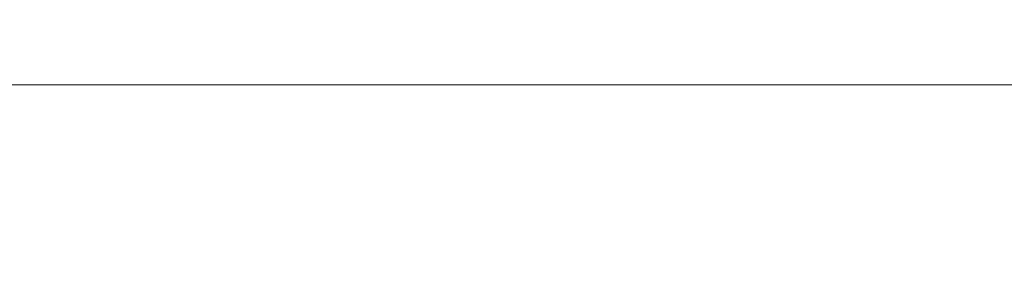
# Model space of a CAD drawing. Units: inches. Extents: x 459864 to 460310, y 324185 to 324787.
# Tile 11 of 112: x 460069.719 to 460071.217, y 324240.835 to 324241.221. Entities that reach past the tile are written whole.
import ezdxf

# ---------------------------------------------------------------- set-up
doc = ezdxf.new("R2010")
doc.units = ezdxf.units.IN
for name, color, linetype, lineweight in [('A-ANNO-DIMS', 2, 'Continuous', 18), ('L-HRDS', 9, 'Continuous', 18), ('L-SITE-PATT', 252, 'Continuous', 13)]:
    doc.layers.add(name, color=color, linetype=linetype, lineweight=lineweight)
doc.styles.get("Standard").update_dxf_attribs({"font": 'arial.ttf'})
doc.dimstyles.new('ISO-25', dxfattribs={"dimtxt": 6, "dimasz": 2.5, "dimexe": 1.25, "dimexo": 0.625, "dimtad": 1, "dimdec": 1, "dimlunit": 3, "dimtxsty": 'Standard', "dimcen": 2.5, "dimadec": 0, "dimazin": 0, "dimtfac": 1, "dimtdec": 1, "dimtmove": 0, "dimatfit": 3, "dimfxl": 1, "dimarcsym": 0})

# ---------------------------------------------------------------- blocks, each defined once
blk = doc.blocks.new('Stepping Stone - hexagonal')
blk.add_line((3.1951, 10.0666), (-5.0989, 10.0666))
blk = doc.blocks.new('*D37')
at = {"layer": 'A-ANNO-DIMS', "color": 0, "lineweight": -2, "transparency": 16777216}
for p, q in [((460077.6779, 324241.1222), (460077.6779, 324260.257)), ((460076.5007, 324241.1222), (460078.9279, 324241.1222)), ((460077.6779, 324231.6078), (460077.6779, 324238.6222)), ((460076.5007, 324229.1078), (460078.9279, 324229.1078))]:
    blk.add_line(p, q, dxfattribs=at)
at = {"layer": 'A-ANNO-DIMS', "color": 0, "transparency": 16777216}
for points in [[(460077.2612, 324238.6222), (460078.0946, 324238.6222), (460077.6779, 324241.1222)], [(460077.2612, 324231.6078), (460078.0946, 324231.6078), (460077.6779, 324229.1078)]]:
    blk.add_solid(points, dxfattribs=at)
at = {"layer": 'Defpoints', "color": 0, "transparency": 16777216}
for p in [(460075.8757, 324241.1222), (460077.6779, 324241.1222), (460075.8757, 324229.1078)]:
    blk.add_point(p, dxfattribs=at)
at = {"layer": 'A-ANNO-DIMS', "color": 0, "transparency": 16777216, "insert": (460073.9895, 324251.9396), "char_height": 6, "attachment_point": 5, "rotation": 90}
blk.add_mtext('1\'-0"', dxfattribs=at)

msp = doc.modelspace()

# ---------------------------------------------------------------- hatches: boundary and pattern name
at = {"layer": 'L-SITE-PATT'}
h = msp.add_hatch(dxfattribs=at)
h.set_pattern_fill('DOTS', color=256)
h.paths.add_polyline_path([(460269.8036, 324283.4832), (460247.1149, 324283.4832), (460121.9293, 324283.4832), (460121.9293, 324252.473), (460117.4293, 324252.473), (460110.1236, 324252.473), (460110.1236, 324243.2865), (460080.8295, 324243.2865), (460080.8295, 324252.473), (460061.1149, 324252.473), (460061.1149, 324251.8824), (460077.9089, 324251.8824), (460077.9089, 324199.4832), (460080.8295, 324199.4832), (460080.8295, 324207.5532), (460110.1236, 324207.5532), (460110.1236, 324199.4832), (460110.8133, 324199.4832), (460262.1149, 324199.4832), (460269.8036, 324199.4832)], flags=17)
edge = h.paths.add_edge_path(flags=0)
edge.add_ellipse((460222.5903, 324263.8132), major_axis=(-8.4853, 8.4853), ratio=1, start_angle=405, end_angle=495, ccw=False)
edge.add_line((460214.8209, 324254.6599), (460214.8316, 324254.6659))
edge.add_ellipse((460222.5903, 324263.8132), major_axis=(-8.4853, 8.4853), ratio=1, start_angle=405, end_angle=495, ccw=False)
edge.add_line((460210.7589, 324261.7806), (460210.7676, 324261.7868))
edge.add_ellipse((460222.5903, 324263.8132), major_axis=(-8.4853, 8.4853), ratio=1, start_angle=405, end_angle=495, ccw=False)
edge.add_ellipse((460222.5903, 324263.8132), major_axis=(-8.4853, 8.4853), ratio=1, start_angle=392.75402, end_angle=405, ccw=False)
edge.add_ellipse((460222.5903, 324263.8132), major_axis=(-8.4853, 8.4853), ratio=1, start_angle=380.93472, end_angle=392.75402, ccw=False)
edge.add_line((460211.3371, 324267.985), (460211.3404, 324267.985))
edge.add_ellipse((460222.5903, 324263.8132), major_axis=(-8.4853, 8.4853), ratio=1, start_angle=380.93472, end_angle=392.75402, ccw=False)
edge.add_ellipse((460222.5903, 324263.8132), major_axis=(-8.4853, 8.4853), ratio=1, start_angle=347.90152, end_angle=380.93472, ccw=False)
edge.add_ellipse((460222.5903, 324263.8132), major_axis=(-8.4853, 8.4853), ratio=1, start_angle=327.06192, end_angle=347.90152, ccw=False)
edge.add_ellipse((460222.5903, 324263.8132), major_axis=(-8.4853, 8.4853), ratio=1, start_angle=278.32464, end_angle=327.06192, ccw=False)
edge.add_line((460225.1583, 324275.536), (460225.1577, 324275.5346))
edge.add_ellipse((460222.5903, 324263.8132), major_axis=(-8.4853, 8.4853), ratio=1, start_angle=278.32464, end_angle=327.06192, ccw=False)
edge.add_ellipse((460222.5903, 324263.8132), major_axis=(-8.4853, 8.4853), ratio=1, start_angle=260.64357, end_angle=278.32464, ccw=False)
edge.add_ellipse((460222.5903, 324263.8132), major_axis=(-8.4853, 8.4853), ratio=1, start_angle=225, end_angle=260.64357, ccw=False)
edge.add_line((460234.5088, 324265.2428), (460234.5015, 324265.2394))
edge.add_ellipse((460222.5903, 324263.8132), major_axis=(-8.4853, 8.4853), ratio=1, start_angle=225, end_angle=260.64357, ccw=False)
edge.add_ellipse((460222.5903, 324263.8132), major_axis=(-8.4853, 8.4853), ratio=1, start_angle=495, end_angle=585, ccw=False)
edge.add_line((460234.4367, 324261.8612), (460234.4238, 324261.8578))
edge.add_ellipse((460222.5903, 324263.8132), major_axis=(-8.4853, 8.4853), ratio=1, start_angle=495, end_angle=585, ccw=False)
edge.add_line((460227.9501, 324253.0672), (460227.9464, 324253.0831))
edge.add_ellipse((460222.5903, 324263.8132), major_axis=(-8.4853, 8.4853), ratio=1, start_angle=495, end_angle=585, ccw=False)
edge.add_line((460226.223, 324252.3693), (460226.211, 324252.3796))
edge.add_ellipse((460222.5903, 324263.8132), major_axis=(-8.4853, 8.4853), ratio=1, start_angle=495, end_angle=585, ccw=False)
h.paths.add_polyline_path([(460219.6515, 324254.3467), (460218.4613, 324253.545), (460218.2754, 324254.7893), (460219.6424, 324256.5418), (460219.6246, 324260.8476), (460216.1101, 324257.333), (460214.35, 324256.9781), (460215.4164, 324259.3557), (460212.5239, 324258.4958), (460213.1373, 324259.9298), (460218.5072, 324263.8132), (460222.5903, 324263.8132), (460222.5903, 324267.8067), (460218.1755, 324272.2123), (460219.026, 324274.639), (460222.5903, 324272.8111), (460222.5903, 324275.4233), (460223.0571, 324274.8249), (460222.6752, 324273.4922), (460225.9117, 324267.1346), (460219.6246, 324260.8476)], flags=0)
edge = h.paths.add_edge_path(flags=0)
edge.add_ellipse((460194.5758, 324264.0465), major_axis=(-8.4853, 8.4853), ratio=1, start_angle=495, end_angle=585, ccw=False)
edge.add_line((460199.9356, 324253.3005), (460199.9319, 324253.3164))
edge.add_ellipse((460194.5758, 324264.0465), major_axis=(-8.4853, 8.4853), ratio=1, start_angle=495, end_angle=585, ccw=False)
edge.add_line((460198.2084, 324252.6025), (460198.1965, 324252.6128))
edge.add_ellipse((460194.5758, 324264.0465), major_axis=(-8.4853, 8.4853), ratio=1, start_angle=495, end_angle=585, ccw=False)
edge.add_ellipse((460194.5758, 324264.0465), major_axis=(-8.4853, 8.4853), ratio=1, start_angle=405, end_angle=495, ccw=False)
edge.add_line((460186.8063, 324254.8932), (460186.8171, 324254.8992))
edge.add_ellipse((460194.5758, 324264.0465), major_axis=(-8.4853, 8.4853), ratio=1, start_angle=405, end_angle=495, ccw=False)
edge.add_line((460182.7444, 324262.0138), (460182.753, 324262.0201))
edge.add_ellipse((460194.5758, 324264.0465), major_axis=(-8.4853, 8.4853), ratio=1, start_angle=405, end_angle=495, ccw=False)
edge.add_ellipse((460194.5758, 324264.0465), major_axis=(-8.4853, 8.4853), ratio=1, start_angle=392.75402, end_angle=405, ccw=False)
edge.add_ellipse((460194.5758, 324264.0465), major_axis=(-8.4853, 8.4853), ratio=1, start_angle=380.93472, end_angle=392.75402, ccw=False)
edge.add_line((460183.3225, 324268.2183), (460183.3259, 324268.2183))
edge.add_ellipse((460194.5758, 324264.0465), major_axis=(-8.4853, 8.4853), ratio=1, start_angle=380.93472, end_angle=392.75402, ccw=False)
edge.add_ellipse((460194.5758, 324264.0465), major_axis=(-8.4853, 8.4853), ratio=1, start_angle=347.90152, end_angle=380.93472, ccw=False)
edge.add_ellipse((460194.5758, 324264.0465), major_axis=(-8.4853, 8.4853), ratio=1, start_angle=327.06192, end_angle=347.90152, ccw=False)
edge.add_ellipse((460194.5758, 324264.0465), major_axis=(-8.4853, 8.4853), ratio=1, start_angle=278.32464, end_angle=327.06192, ccw=False)
edge.add_line((460197.1437, 324275.7693), (460197.1432, 324275.7679))
edge.add_ellipse((460194.5758, 324264.0465), major_axis=(-8.4853, 8.4853), ratio=1, start_angle=278.32464, end_angle=327.06192, ccw=False)
edge.add_ellipse((460194.5758, 324264.0465), major_axis=(-8.4853, 8.4853), ratio=1, start_angle=260.64357, end_angle=278.32464, ccw=False)
edge.add_ellipse((460194.5758, 324264.0465), major_axis=(-8.4853, 8.4853), ratio=1, start_angle=225, end_angle=260.64357, ccw=False)
edge.add_line((460206.4943, 324265.4761), (460206.4869, 324265.4727))
edge.add_ellipse((460194.5758, 324264.0465), major_axis=(-8.4853, 8.4853), ratio=1, start_angle=225, end_angle=260.64357, ccw=False)
edge.add_ellipse((460194.5758, 324264.0465), major_axis=(-8.4853, 8.4853), ratio=1, start_angle=495, end_angle=585, ccw=False)
edge.add_line((460206.4221, 324262.0945), (460206.4092, 324262.0911))
h.paths.add_polyline_path([(460191.6101, 324261.0808), (460191.6369, 324254.5799), (460190.4468, 324253.7783), (460190.2609, 324255.0226), (460191.6279, 324256.775), (460191.6101, 324261.0808), (460188.0956, 324257.5663), (460186.3354, 324257.2113), (460187.4018, 324259.5889), (460184.5094, 324258.7291), (460185.1228, 324260.1631), (460190.4927, 324264.0465), (460194.5758, 324264.0465), (460194.5758, 324268.04), (460190.161, 324272.4456), (460191.0114, 324274.8722), (460194.5758, 324273.0444), (460194.5758, 324275.6566), (460195.0426, 324275.0582), (460194.6607, 324273.7255), (460197.8971, 324267.3679)], flags=0)
edge = h.paths.add_edge_path(flags=0)
edge.add_ellipse((460252.912, 324263.5776), major_axis=(-8.4853, 8.4853), ratio=1, start_angle=405, end_angle=495, ccw=False)
edge.add_line((460241.0806, 324261.5449), (460241.0892, 324261.5512))
edge.add_ellipse((460252.912, 324263.5776), major_axis=(-8.4853, 8.4853), ratio=1, start_angle=405, end_angle=495, ccw=False)
edge.add_ellipse((460252.912, 324263.5776), major_axis=(-8.4853, 8.4853), ratio=1, start_angle=392.75402, end_angle=405, ccw=False)
edge.add_ellipse((460252.912, 324263.5776), major_axis=(-8.4853, 8.4853), ratio=1, start_angle=380.93472, end_angle=392.75402, ccw=False)
edge.add_line((460241.6587, 324267.7494), (460241.6621, 324267.7494))
edge.add_ellipse((460252.912, 324263.5776), major_axis=(-8.4853, 8.4853), ratio=1, start_angle=380.93472, end_angle=392.75402, ccw=False)
edge.add_ellipse((460252.912, 324263.5776), major_axis=(-8.4853, 8.4853), ratio=1, start_angle=347.90152, end_angle=380.93472, ccw=False)
edge.add_ellipse((460252.912, 324263.5776), major_axis=(-8.4853, 8.4853), ratio=1, start_angle=327.06192, end_angle=347.90152, ccw=False)
edge.add_ellipse((460252.912, 324263.5776), major_axis=(-8.4853, 8.4853), ratio=1, start_angle=278.32464, end_angle=327.06192, ccw=False)
edge.add_line((460255.4799, 324275.3004), (460255.4794, 324275.299))
edge.add_ellipse((460252.912, 324263.5776), major_axis=(-8.4853, 8.4853), ratio=1, start_angle=278.32464, end_angle=327.06192, ccw=False)
edge.add_ellipse((460252.912, 324263.5776), major_axis=(-8.4853, 8.4853), ratio=1, start_angle=260.64357, end_angle=278.32464, ccw=False)
edge.add_ellipse((460252.912, 324263.5776), major_axis=(-8.4853, 8.4853), ratio=1, start_angle=225, end_angle=260.64357, ccw=False)
edge.add_line((460264.8305, 324265.0072), (460264.8231, 324265.0038))
edge.add_ellipse((460252.912, 324263.5776), major_axis=(-8.4853, 8.4853), ratio=1, start_angle=225, end_angle=260.64357, ccw=False)
edge.add_ellipse((460252.912, 324263.5776), major_axis=(-8.4853, 8.4853), ratio=1, start_angle=495, end_angle=585, ccw=False)
edge.add_line((460264.7583, 324261.6256), (460264.7454, 324261.6222))
edge.add_ellipse((460252.912, 324263.5776), major_axis=(-8.4853, 8.4853), ratio=1, start_angle=495, end_angle=585, ccw=False)
edge.add_line((460258.2718, 324252.8316), (460258.2681, 324252.8475))
edge.add_ellipse((460252.912, 324263.5776), major_axis=(-8.4853, 8.4853), ratio=1, start_angle=495, end_angle=585, ccw=False)
edge.add_line((460256.5446, 324252.1337), (460256.5327, 324252.1439))
edge.add_ellipse((460252.912, 324263.5776), major_axis=(-8.4853, 8.4853), ratio=1, start_angle=495, end_angle=585, ccw=False)
edge.add_ellipse((460252.912, 324263.5776), major_axis=(-8.4853, 8.4853), ratio=1, start_angle=405, end_angle=495, ccw=False)
edge.add_line((460245.1425, 324254.4243), (460245.1533, 324254.4303))
h.paths.add_polyline_path([(460244.6716, 324256.7425), (460245.738, 324259.1201), (460242.8456, 324258.2602), (460243.459, 324259.6942), (460248.8289, 324263.5776), (460252.912, 324263.5776), (460252.912, 324267.5711), (460248.4972, 324271.9767), (460249.3476, 324274.4034), (460252.912, 324272.5755), (460252.912, 324275.1877), (460253.3788, 324274.5893), (460252.9969, 324273.2566), (460256.2333, 324266.899), (460249.9463, 324260.612), (460249.9731, 324254.111), (460248.783, 324253.3094), (460248.5971, 324254.5537), (460249.9641, 324256.3062), (460249.9463, 324260.612), (460246.4318, 324257.0974)], flags=0)
edge = h.paths.add_edge_path(flags=0)
edge.add_ellipse((460167.4387, 324262.8328), major_axis=(-8.4853, 8.4853), ratio=1, start_angle=495, end_angle=585, ccw=False)
edge.add_line((460172.7985, 324252.0868), (460172.7948, 324252.1027))
edge.add_ellipse((460167.4387, 324262.8328), major_axis=(-8.4853, 8.4853), ratio=1, start_angle=495, end_angle=585, ccw=False)
edge.add_line((460171.0714, 324251.3888), (460171.0594, 324251.3991))
edge.add_ellipse((460167.4387, 324262.8328), major_axis=(-8.4853, 8.4853), ratio=1, start_angle=495, end_angle=585, ccw=False)
edge.add_ellipse((460167.4387, 324262.8328), major_axis=(-8.4853, 8.4853), ratio=1, start_angle=405, end_angle=495, ccw=False)
edge.add_line((460159.6693, 324253.6795), (460159.68, 324253.6855))
edge.add_ellipse((460167.4387, 324262.8328), major_axis=(-8.4853, 8.4853), ratio=1, start_angle=405, end_angle=495, ccw=False)
edge.add_line((460155.6073, 324260.8001), (460155.616, 324260.8064))
edge.add_ellipse((460167.4387, 324262.8328), major_axis=(-8.4853, 8.4853), ratio=1, start_angle=405, end_angle=495, ccw=False)
edge.add_ellipse((460167.4387, 324262.8328), major_axis=(-8.4853, 8.4853), ratio=1, start_angle=392.75402, end_angle=405, ccw=False)
edge.add_ellipse((460167.4387, 324262.8328), major_axis=(-8.4853, 8.4853), ratio=1, start_angle=380.93472, end_angle=392.75402, ccw=False)
edge.add_line((460156.1855, 324267.0046), (460156.1888, 324267.0046))
edge.add_ellipse((460167.4387, 324262.8328), major_axis=(-8.4853, 8.4853), ratio=1, start_angle=380.93472, end_angle=392.75402, ccw=False)
edge.add_ellipse((460167.4387, 324262.8328), major_axis=(-8.4853, 8.4853), ratio=1, start_angle=347.90152, end_angle=380.93472, ccw=False)
edge.add_ellipse((460167.4387, 324262.8328), major_axis=(-8.4853, 8.4853), ratio=1, start_angle=327.06192, end_angle=347.90152, ccw=False)
edge.add_ellipse((460167.4387, 324262.8328), major_axis=(-8.4853, 8.4853), ratio=1, start_angle=278.32464, end_angle=327.06192, ccw=False)
edge.add_line((460170.0067, 324274.5556), (460170.0061, 324274.5542))
edge.add_ellipse((460167.4387, 324262.8328), major_axis=(-8.4853, 8.4853), ratio=1, start_angle=278.32464, end_angle=327.06192, ccw=False)
edge.add_ellipse((460167.4387, 324262.8328), major_axis=(-8.4853, 8.4853), ratio=1, start_angle=260.64357, end_angle=278.32464, ccw=False)
edge.add_ellipse((460167.4387, 324262.8328), major_axis=(-8.4853, 8.4853), ratio=1, start_angle=225, end_angle=260.64357, ccw=False)
edge.add_line((460179.3572, 324264.2624), (460179.3499, 324264.259))
edge.add_ellipse((460167.4387, 324262.8328), major_axis=(-8.4853, 8.4853), ratio=1, start_angle=225, end_angle=260.64357, ccw=False)
edge.add_ellipse((460167.4387, 324262.8328), major_axis=(-8.4853, 8.4853), ratio=1, start_angle=495, end_angle=585, ccw=False)
edge.add_line((460179.2851, 324260.8808), (460179.2722, 324260.8774))
h.paths.add_polyline_path([(460164.473, 324259.8671), (460164.4998, 324253.3662), (460163.3097, 324252.5645), (460163.1238, 324253.8089), (460164.4908, 324255.5613), (460164.473, 324259.8671), (460160.9585, 324256.3526), (460159.1984, 324255.9976), (460160.2648, 324258.3752), (460157.3723, 324257.5154), (460157.9857, 324258.9494), (460163.3556, 324262.8328), (460167.4387, 324262.8328), (460167.4387, 324266.8263), (460163.0239, 324271.2319), (460163.8744, 324273.6585), (460167.4387, 324271.8307), (460167.4387, 324274.4429), (460167.9055, 324273.8445), (460167.5236, 324272.5118), (460170.7601, 324266.1542)], flags=0)
edge = h.paths.add_edge_path(flags=0)
edge.add_ellipse((460140.7581, 324262.3696), major_axis=(-8.4853, 8.4853), ratio=1, start_angle=495, end_angle=585, ccw=False)
edge.add_line((460146.1179, 324251.6235), (460146.1142, 324251.6395))
edge.add_ellipse((460140.7581, 324262.3696), major_axis=(-8.4853, 8.4853), ratio=1, start_angle=495, end_angle=585, ccw=False)
edge.add_line((460144.3908, 324250.9256), (460144.3788, 324250.9359))
edge.add_ellipse((460140.7581, 324262.3696), major_axis=(-8.4853, 8.4853), ratio=1, start_angle=495, end_angle=585, ccw=False)
edge.add_ellipse((460140.7581, 324262.3696), major_axis=(-8.4853, 8.4853), ratio=1, start_angle=405, end_angle=495, ccw=False)
edge.add_line((460132.9887, 324253.2162), (460132.9994, 324253.2223))
edge.add_ellipse((460140.7581, 324262.3696), major_axis=(-8.4853, 8.4853), ratio=1, start_angle=405, end_angle=495, ccw=False)
edge.add_line((460128.9267, 324260.3369), (460128.9354, 324260.3432))
edge.add_ellipse((460140.7581, 324262.3696), major_axis=(-8.4853, 8.4853), ratio=1, start_angle=405, end_angle=495, ccw=False)
edge.add_ellipse((460140.7581, 324262.3696), major_axis=(-8.4853, 8.4853), ratio=1, start_angle=392.75402, end_angle=405, ccw=False)
edge.add_ellipse((460140.7581, 324262.3696), major_axis=(-8.4853, 8.4853), ratio=1, start_angle=380.93472, end_angle=392.75402, ccw=False)
edge.add_line((460129.5049, 324266.5414), (460129.5082, 324266.5414))
edge.add_ellipse((460140.7581, 324262.3696), major_axis=(-8.4853, 8.4853), ratio=1, start_angle=380.93472, end_angle=392.75402, ccw=False)
edge.add_ellipse((460140.7581, 324262.3696), major_axis=(-8.4853, 8.4853), ratio=1, start_angle=347.90152, end_angle=380.93472, ccw=False)
edge.add_ellipse((460140.7581, 324262.3696), major_axis=(-8.4853, 8.4853), ratio=1, start_angle=327.06192, end_angle=347.90152, ccw=False)
edge.add_ellipse((460140.7581, 324262.3696), major_axis=(-8.4853, 8.4853), ratio=1, start_angle=278.32464, end_angle=327.06192, ccw=False)
edge.add_line((460143.3261, 324274.0923), (460143.3255, 324274.091))
edge.add_ellipse((460140.7581, 324262.3696), major_axis=(-8.4853, 8.4853), ratio=1, start_angle=278.32464, end_angle=327.06192, ccw=False)
edge.add_ellipse((460140.7581, 324262.3696), major_axis=(-8.4853, 8.4853), ratio=1, start_angle=260.64357, end_angle=278.32464, ccw=False)
edge.add_ellipse((460140.7581, 324262.3696), major_axis=(-8.4853, 8.4853), ratio=1, start_angle=225, end_angle=260.64357, ccw=False)
edge.add_line((460152.6766, 324263.7992), (460152.6692, 324263.7958))
edge.add_ellipse((460140.7581, 324262.3696), major_axis=(-8.4853, 8.4853), ratio=1, start_angle=225, end_angle=260.64357, ccw=False)
edge.add_ellipse((460140.7581, 324262.3696), major_axis=(-8.4853, 8.4853), ratio=1, start_angle=495, end_angle=585, ccw=False)
edge.add_line((460152.6045, 324260.4176), (460152.5916, 324260.4142))
h.paths.add_polyline_path([(460137.7924, 324259.4039), (460137.8192, 324252.903), (460136.6291, 324252.1013), (460136.4432, 324253.3457), (460137.8102, 324255.0981), (460137.7924, 324259.4039), (460134.2779, 324255.8894), (460132.5178, 324255.5344), (460133.5842, 324257.912), (460130.6917, 324257.0522), (460131.3051, 324258.4862), (460136.675, 324262.3696), (460140.7581, 324262.3696), (460140.7581, 324266.3631), (460136.3433, 324270.7687), (460137.1938, 324273.1953), (460140.7581, 324271.3675), (460140.7581, 324273.9797), (460141.2249, 324273.3813), (460140.843, 324272.0486), (460144.0795, 324265.691)], flags=0)
h.paths.add_polyline_path([(460110.1236, 324227.4139), (460080.8295, 324227.4139), (460080.8295, 324235.4839), (460110.1236, 324235.4839)], flags=16)
h.paths.add_polyline_path([(460110.1236, 324220.7966), (460110.1236, 324212.7267), (460080.8295, 324212.7267), (460080.8295, 324220.7966)], flags=16)
h.paths.add_polyline_path([(460269.8036, 324283.4832), (460247.1149, 324283.4832), (460121.9293, 324283.4832), (460121.9293, 324252.473), (460117.4293, 324252.473), (460110.1236, 324252.473), (460110.1236, 324243.2865), (460080.8295, 324243.2865), (460080.8295, 324252.473), (460061.1149, 324252.473), (460061.1149, 324251.8824), (460077.9089, 324251.8824), (460077.9089, 324199.4832), (460080.8295, 324199.4832), (460080.8295, 324207.5532), (460110.1236, 324207.5532), (460110.1236, 324199.4832), (460262.1149, 324199.4832), (460269.8036, 324199.4832)], flags=17)
h.paths.add_polyline_path([(460219.6515, 324254.3467), (460218.4613, 324253.545), (460218.2754, 324254.7893), (460219.6424, 324256.5418), (460219.6246, 324260.8476), (460216.1101, 324257.333), (460214.35, 324256.9781), (460215.4164, 324259.3557), (460212.5239, 324258.4958), (460213.1373, 324259.9298), (460218.5072, 324263.8132), (460222.5903, 324263.8132), (460220.1805, 324266.223), (460215.461, 324265.3076), (460211.8345, 324266.1366), (460216.2466, 324267.985), (460218.4185, 324267.985), (460222.5903, 324263.8132), (460222.5903, 324267.8067), (460218.1755, 324272.2123), (460219.026, 324274.639), (460222.5903, 324272.8111), (460222.5903, 324275.4233), (460223.0571, 324274.8249), (460222.6752, 324273.4922), (460225.9117, 324267.1346), (460222.5903, 324263.8132), (460231.3829, 324263.8132), (460228.4847, 324262.4878), (460224.4252, 324261.9783), (460228.6799, 324257.7236), (460228.9658, 324254.791), (460227.1418, 324256.5366), (460227.5421, 324254.8186), (460227.3333, 324253.6145), (460222.5903, 324259.9846), (460222.5903, 324255.4967), (460221.3774, 324256.5408), (460220.5758, 324261.7987), (460219.6246, 324260.8476)], flags=0)
h.paths.add_polyline_path([(460199.1272, 324256.7699), (460199.5275, 324255.0518), (460199.3188, 324253.8477), (460194.5758, 324260.2179), (460194.5758, 324255.7299), (460193.3629, 324256.7741), (460192.5613, 324262.032), (460191.6101, 324261.0808), (460191.6369, 324254.5799), (460190.4468, 324253.7783), (460190.2609, 324255.0226), (460191.6279, 324256.775), (460191.6101, 324261.0808), (460188.0956, 324257.5663), (460186.3354, 324257.2113), (460187.4018, 324259.5889), (460184.5094, 324258.7291), (460185.1228, 324260.1631), (460190.4927, 324264.0465), (460194.5758, 324264.0465), (460192.1659, 324266.4563), (460187.4464, 324265.5409), (460183.82, 324266.3698), (460188.2321, 324268.2183), (460190.404, 324268.2183), (460194.5758, 324264.0465), (460194.5758, 324268.04), (460190.161, 324272.4456), (460191.0114, 324274.8722), (460194.5758, 324273.0444), (460194.5758, 324275.6566), (460195.0426, 324275.0582), (460194.6607, 324273.7255), (460197.8971, 324267.3679), (460194.5758, 324264.0465), (460203.3683, 324264.0465), (460200.4702, 324262.7211), (460196.4107, 324262.2116), (460200.6654, 324257.9569), (460200.9513, 324255.0243)], flags=0)
h.paths.add_polyline_path([(460244.6716, 324256.7425), (460245.738, 324259.1201), (460242.8456, 324258.2602), (460243.459, 324259.6942), (460248.8289, 324263.5776), (460252.912, 324263.5776), (460250.5022, 324265.9874), (460245.7826, 324265.072), (460242.1562, 324265.9009), (460246.5683, 324267.7494), (460248.7402, 324267.7494), (460252.912, 324263.5776), (460252.912, 324267.5711), (460248.4972, 324271.9767), (460249.3476, 324274.4034), (460252.912, 324272.5755), (460252.912, 324275.1877), (460253.3788, 324274.5893), (460252.9969, 324273.2566), (460256.2333, 324266.899), (460252.912, 324263.5776), (460261.7045, 324263.5776), (460258.8064, 324262.2522), (460254.7469, 324261.7427), (460259.0016, 324257.488), (460259.2875, 324254.5554), (460257.4634, 324256.301), (460257.8637, 324254.583), (460257.655, 324253.3789), (460252.912, 324259.749), (460252.912, 324255.2611), (460251.6991, 324256.3052), (460250.8975, 324261.5631), (460249.9463, 324260.612), (460249.9731, 324254.111), (460248.783, 324253.3094), (460248.5971, 324254.5537), (460249.9641, 324256.3062), (460249.9463, 324260.612), (460246.4318, 324257.0974)], flags=0)
h.paths.add_polyline_path([(460173.5283, 324256.7432), (460173.8142, 324253.8106), (460171.9902, 324255.5562), (460172.3905, 324253.8381), (460172.1817, 324252.634), (460167.4387, 324259.0042), (460167.4387, 324254.5162), (460166.2258, 324255.5604), (460165.4242, 324260.8183), (460164.473, 324259.8671), (460164.4998, 324253.3662), (460163.3097, 324252.5645), (460163.1238, 324253.8089), (460164.4908, 324255.5613), (460164.473, 324259.8671), (460160.9585, 324256.3526), (460159.1984, 324255.9976), (460160.2648, 324258.3752), (460157.3723, 324257.5154), (460157.9857, 324258.9494), (460163.3556, 324262.8328), (460167.4387, 324262.8328), (460165.0289, 324265.2426), (460160.3094, 324264.3272), (460156.6829, 324265.1561), (460161.095, 324267.0046), (460163.2669, 324267.0046), (460167.4387, 324262.8328), (460167.4387, 324266.8263), (460163.0239, 324271.2319), (460163.8744, 324273.6585), (460167.4387, 324271.8307), (460167.4387, 324274.4429), (460167.9055, 324273.8445), (460167.5236, 324272.5118), (460170.7601, 324266.1542), (460167.4387, 324262.8328), (460176.2313, 324262.8328), (460173.3331, 324261.5074), (460169.2736, 324260.9979)], flags=0)
h.paths.add_polyline_path([(460146.8477, 324256.28), (460147.1336, 324253.3474), (460145.3096, 324255.093), (460145.7099, 324253.3749), (460145.5011, 324252.1708), (460140.7581, 324258.541), (460140.7581, 324254.053), (460139.5452, 324255.0972), (460138.7436, 324260.3551), (460137.7924, 324259.4039), (460137.8192, 324252.903), (460136.6291, 324252.1013), (460136.4432, 324253.3457), (460137.8102, 324255.0981), (460137.7924, 324259.4039), (460134.2779, 324255.8894), (460132.5178, 324255.5344), (460133.5842, 324257.912), (460130.6917, 324257.0522), (460131.3051, 324258.4862), (460136.675, 324262.3696), (460140.7581, 324262.3696), (460138.3483, 324264.7794), (460133.6288, 324263.864), (460130.0023, 324264.6929), (460134.4144, 324266.5414), (460136.5863, 324266.5414), (460140.7581, 324262.3696), (460140.7581, 324266.3631), (460136.3433, 324270.7687), (460137.1938, 324273.1953), (460140.7581, 324271.3675), (460140.7581, 324273.9797), (460141.2249, 324273.3813), (460140.843, 324272.0486), (460144.0795, 324265.691), (460140.7581, 324262.3696), (460149.5507, 324262.3696), (460146.6525, 324261.0442), (460142.593, 324260.5347)], flags=0)
edge = h.paths.add_edge_path()
edge.add_line((460269.8036, 324272.5491), (460260.8815, 324272.5491))
edge.add_ellipse((460252.912, 324263.5776), major_axis=(-8.4853, 8.4853), ratio=1, start_angle=260.64357, end_angle=273.38462, ccw=False)
edge.add_line((460262.2826, 324271.0921), (460262.2606, 324271.0911))
edge.add_ellipse((460252.912, 324263.5776), major_axis=(-8.4853, 8.4853), ratio=1, start_angle=260.64357, end_angle=273.38462, ccw=False)
edge.add_ellipse((460252.912, 324263.5776), major_axis=(-8.4853, 8.4853), ratio=1, start_angle=225, end_angle=260.64357, ccw=False)
edge.add_line((460263.6086, 324269.0633), (460263.5717, 324269.0583))
edge.add_ellipse((460252.912, 324263.5776), major_axis=(-8.4853, 8.4853), ratio=1, start_angle=225, end_angle=260.64357, ccw=False)
edge.add_line((460264.6155, 324266.3055), (460264.5854, 324266.3052))
edge.add_ellipse((460252.912, 324263.5776), major_axis=(-8.4853, 8.4853), ratio=1, start_angle=225, end_angle=260.64357, ccw=False)
edge.add_line((460264.8305, 324265.0072), (460264.8231, 324265.0038))
edge.add_ellipse((460252.912, 324263.5776), major_axis=(-8.4853, 8.4853), ratio=1, start_angle=225, end_angle=260.64357, ccw=False)
edge.add_ellipse((460252.912, 324263.5776), major_axis=(-8.4853, 8.4853), ratio=1, start_angle=495, end_angle=585, ccw=False)
edge.add_line((460264.7583, 324261.6256), (460264.7454, 324261.6222))
edge.add_ellipse((460252.912, 324263.5776), major_axis=(-8.4853, 8.4853), ratio=1, start_angle=495, end_angle=585, ccw=False)
edge.add_line((460263.4422, 324257.739), (460263.3893, 324257.7792))
edge.add_ellipse((460252.912, 324263.5776), major_axis=(-8.4853, 8.4853), ratio=1, start_angle=495, end_angle=585, ccw=False)
edge.add_line((460258.1281, 324252.7435), (460258.1019, 324252.7787))
edge.add_ellipse((460252.912, 324263.5776), major_axis=(-8.4853, 8.4853), ratio=1, start_angle=495, end_angle=585, ccw=False)
edge.add_line((460256.5446, 324252.1337), (460256.5327, 324252.1439))
edge.add_ellipse((460252.912, 324263.5776), major_axis=(-8.4853, 8.4853), ratio=1, start_angle=495, end_angle=585, ccw=False)
edge.add_ellipse((460252.912, 324263.5776), major_axis=(-8.4853, 8.4853), ratio=1, start_angle=405, end_angle=495, ccw=False)
edge.add_line((460250.594, 324251.7804), (460250.6047, 324251.8198))
edge.add_ellipse((460252.912, 324263.5776), major_axis=(-8.4853, 8.4853), ratio=1, start_angle=405, end_angle=495, ccw=False)
edge.add_line((460245.1425, 324254.4243), (460245.1533, 324254.4303))
edge.add_ellipse((460252.912, 324263.5776), major_axis=(-8.4853, 8.4853), ratio=1, start_angle=405, end_angle=495, ccw=False)
edge.add_line((460243.5246, 324256.059), (460243.5603, 324256.0914))
edge.add_ellipse((460252.912, 324263.5776), major_axis=(-8.4853, 8.4853), ratio=1, start_angle=405, end_angle=495, ccw=False)
edge.add_line((460241.4401, 324259.8927), (460241.5224, 324259.8959))
edge.add_ellipse((460252.912, 324263.5776), major_axis=(-8.4853, 8.4853), ratio=1, start_angle=405, end_angle=495, ccw=False)
edge.add_line((460241.0806, 324261.5449), (460241.0892, 324261.5512))
edge.add_ellipse((460252.912, 324263.5776), major_axis=(-8.4853, 8.4853), ratio=1, start_angle=405, end_angle=495, ccw=False)
edge.add_ellipse((460252.912, 324263.5776), major_axis=(-8.4853, 8.4853), ratio=1, start_angle=392.75402, end_angle=405, ccw=False)
edge.add_line((460241.0503, 324265.4376), (460241.0626, 324265.4428))
edge.add_ellipse((460252.912, 324263.5776), major_axis=(-8.4853, 8.4853), ratio=1, start_angle=392.75402, end_angle=405, ccw=False)
edge.add_ellipse((460252.912, 324263.5776), major_axis=(-8.4853, 8.4853), ratio=1, start_angle=380.93472, end_angle=392.75402, ccw=False)
edge.add_line((460241.4519, 324267.1764), (460241.469, 324267.171))
edge.add_ellipse((460252.912, 324263.5776), major_axis=(-8.4853, 8.4853), ratio=1, start_angle=380.93472, end_angle=392.75402, ccw=False)
edge.add_line((460241.6587, 324267.7494), (460241.6621, 324267.7494))
edge.add_ellipse((460252.912, 324263.5776), major_axis=(-8.4853, 8.4853), ratio=1, start_angle=380.93472, end_angle=392.75402, ccw=False)
edge.add_ellipse((460252.912, 324263.5776), major_axis=(-8.4853, 8.4853), ratio=1, start_angle=356.61538, end_angle=380.93472, ccw=False)
edge.add_line((460244.8803, 324272.4877), (460244.7127, 324272.5491))
edge.add_line((460244.7127, 324272.5491), (460230.8174, 324272.5491))
edge.add_ellipse((460222.5903, 324263.8132), major_axis=(-8.4853, 8.4853), ratio=1, start_angle=260.64357, end_angle=271.71777, ccw=False)
edge.add_ellipse((460222.5903, 324263.8132), major_axis=(-8.4853, 8.4853), ratio=1, start_angle=225, end_angle=260.64357, ccw=False)
edge.add_line((460233.2869, 324269.2989), (460233.25, 324269.2939))
edge.add_ellipse((460222.5903, 324263.8132), major_axis=(-8.4853, 8.4853), ratio=1, start_angle=225, end_angle=260.64357, ccw=False)
edge.add_line((460234.2938, 324266.5412), (460234.2637, 324266.5408))
edge.add_ellipse((460222.5903, 324263.8132), major_axis=(-8.4853, 8.4853), ratio=1, start_angle=225, end_angle=260.64357, ccw=False)
edge.add_line((460234.5088, 324265.2428), (460234.5015, 324265.2394))
edge.add_ellipse((460222.5903, 324263.8132), major_axis=(-8.4853, 8.4853), ratio=1, start_angle=225, end_angle=260.64357, ccw=False)
edge.add_ellipse((460222.5903, 324263.8132), major_axis=(-8.4853, 8.4853), ratio=1, start_angle=495, end_angle=585, ccw=False)
edge.add_line((460234.4367, 324261.8612), (460234.4238, 324261.8578))
edge.add_ellipse((460222.5903, 324263.8132), major_axis=(-8.4853, 8.4853), ratio=1, start_angle=495, end_angle=585, ccw=False)
edge.add_line((460233.1205, 324257.9746), (460233.0676, 324258.0149))
edge.add_ellipse((460222.5903, 324263.8132), major_axis=(-8.4853, 8.4853), ratio=1, start_angle=495, end_angle=585, ccw=False)
edge.add_line((460227.8064, 324252.9791), (460227.7802, 324253.0143))
edge.add_ellipse((460222.5903, 324263.8132), major_axis=(-8.4853, 8.4853), ratio=1, start_angle=495, end_angle=585, ccw=False)
edge.add_line((460226.223, 324252.3693), (460226.211, 324252.3796))
edge.add_ellipse((460222.5903, 324263.8132), major_axis=(-8.4853, 8.4853), ratio=1, start_angle=495, end_angle=585, ccw=False)
edge.add_ellipse((460222.5903, 324263.8132), major_axis=(-8.4853, 8.4853), ratio=1, start_angle=405, end_angle=495, ccw=False)
edge.add_line((460220.2723, 324252.016), (460220.283, 324252.0554))
edge.add_ellipse((460222.5903, 324263.8132), major_axis=(-8.4853, 8.4853), ratio=1, start_angle=405, end_angle=495, ccw=False)
edge.add_line((460214.8209, 324254.6599), (460214.8316, 324254.6659))
edge.add_ellipse((460222.5903, 324263.8132), major_axis=(-8.4853, 8.4853), ratio=1, start_angle=405, end_angle=495, ccw=False)
edge.add_line((460213.2029, 324256.2946), (460213.2387, 324256.327))
edge.add_ellipse((460222.5903, 324263.8132), major_axis=(-8.4853, 8.4853), ratio=1, start_angle=405, end_angle=495, ccw=False)
edge.add_line((460211.1184, 324260.1283), (460211.2008, 324260.1315))
edge.add_ellipse((460222.5903, 324263.8132), major_axis=(-8.4853, 8.4853), ratio=1, start_angle=405, end_angle=495, ccw=False)
edge.add_line((460210.7589, 324261.7806), (460210.7676, 324261.7868))
edge.add_ellipse((460222.5903, 324263.8132), major_axis=(-8.4853, 8.4853), ratio=1, start_angle=405, end_angle=495, ccw=False)
edge.add_ellipse((460222.5903, 324263.8132), major_axis=(-8.4853, 8.4853), ratio=1, start_angle=392.75402, end_angle=405, ccw=False)
edge.add_line((460210.7286, 324265.6732), (460210.7409, 324265.6784))
edge.add_ellipse((460222.5903, 324263.8132), major_axis=(-8.4853, 8.4853), ratio=1, start_angle=392.75402, end_angle=405, ccw=False)
edge.add_ellipse((460222.5903, 324263.8132), major_axis=(-8.4853, 8.4853), ratio=1, start_angle=380.93472, end_angle=392.75402, ccw=False)
edge.add_line((460211.1302, 324267.412), (460211.1474, 324267.4066))
edge.add_ellipse((460222.5903, 324263.8132), major_axis=(-8.4853, 8.4853), ratio=1, start_angle=380.93472, end_angle=392.75402, ccw=False)
edge.add_line((460211.3371, 324267.985), (460211.3404, 324267.985))
edge.add_ellipse((460222.5903, 324263.8132), major_axis=(-8.4853, 8.4853), ratio=1, start_angle=380.93472, end_angle=392.75402, ccw=False)
edge.add_ellipse((460222.5903, 324263.8132), major_axis=(-8.4853, 8.4853), ratio=1, start_angle=358.28223, end_angle=380.93472, ccw=False)
edge.add_line((460213.7045, 324271.9018), (460213.709, 324271.869))
edge.add_ellipse((460222.5903, 324263.8132), major_axis=(-8.4853, 8.4853), ratio=1, start_angle=358.28223, end_angle=380.93472, ccw=False)
edge.add_line((460214.3632, 324272.5491), (460203.0783, 324272.5491))
edge.add_line((460203.0783, 324272.5491), (460203.0603, 324272.5311))
edge.add_ellipse((460194.5758, 324264.0465), major_axis=(-8.4853, 8.4853), ratio=1, start_angle=260.64357, end_angle=270.11679, ccw=False)
edge.add_line((460203.9566, 324271.5615), (460203.9209, 324271.5598))
edge.add_ellipse((460194.5758, 324264.0465), major_axis=(-8.4853, 8.4853), ratio=1, start_angle=260.64357, end_angle=270.11679, ccw=False)
edge.add_ellipse((460194.5758, 324264.0465), major_axis=(-8.4853, 8.4853), ratio=1, start_angle=225, end_angle=260.64357, ccw=False)
edge.add_line((460205.2724, 324269.5322), (460205.2354, 324269.5272))
edge.add_ellipse((460194.5758, 324264.0465), major_axis=(-8.4853, 8.4853), ratio=1, start_angle=225, end_angle=260.64357, ccw=False)
edge.add_line((460206.2793, 324266.7744), (460206.2492, 324266.7741))
edge.add_ellipse((460194.5758, 324264.0465), major_axis=(-8.4853, 8.4853), ratio=1, start_angle=225, end_angle=260.64357, ccw=False)
edge.add_line((460206.4943, 324265.4761), (460206.4869, 324265.4727))
edge.add_ellipse((460194.5758, 324264.0465), major_axis=(-8.4853, 8.4853), ratio=1, start_angle=225, end_angle=260.64357, ccw=False)
edge.add_ellipse((460194.5758, 324264.0465), major_axis=(-8.4853, 8.4853), ratio=1, start_angle=495, end_angle=585, ccw=False)
edge.add_line((460206.4221, 324262.0945), (460206.4092, 324262.0911))
edge.add_ellipse((460194.5758, 324264.0465), major_axis=(-8.4853, 8.4853), ratio=1, start_angle=495, end_angle=585, ccw=False)
edge.add_line((460205.106, 324258.2079), (460205.0531, 324258.2481))
edge.add_ellipse((460194.5758, 324264.0465), major_axis=(-8.4853, 8.4853), ratio=1, start_angle=495, end_angle=585, ccw=False)
edge.add_line((460199.7919, 324253.2124), (460199.7657, 324253.2476))
edge.add_ellipse((460194.5758, 324264.0465), major_axis=(-8.4853, 8.4853), ratio=1, start_angle=495, end_angle=585, ccw=False)
edge.add_line((460198.2084, 324252.6025), (460198.1965, 324252.6128))
edge.add_ellipse((460194.5758, 324264.0465), major_axis=(-8.4853, 8.4853), ratio=1, start_angle=495, end_angle=585, ccw=False)
edge.add_ellipse((460194.5758, 324264.0465), major_axis=(-8.4853, 8.4853), ratio=1, start_angle=405, end_angle=495, ccw=False)
edge.add_line((460192.2578, 324252.2493), (460192.2684, 324252.2887))
edge.add_ellipse((460194.5758, 324264.0465), major_axis=(-8.4853, 8.4853), ratio=1, start_angle=405, end_angle=495, ccw=False)
edge.add_line((460186.8063, 324254.8932), (460186.8171, 324254.8992))
edge.add_ellipse((460194.5758, 324264.0465), major_axis=(-8.4853, 8.4853), ratio=1, start_angle=405, end_angle=495, ccw=False)
edge.add_line((460185.1884, 324256.5279), (460185.2241, 324256.5602))
edge.add_ellipse((460194.5758, 324264.0465), major_axis=(-8.4853, 8.4853), ratio=1, start_angle=405, end_angle=495, ccw=False)
edge.add_line((460183.1039, 324260.3616), (460183.1862, 324260.3648))
edge.add_ellipse((460194.5758, 324264.0465), major_axis=(-8.4853, 8.4853), ratio=1, start_angle=405, end_angle=495, ccw=False)
edge.add_line((460182.7444, 324262.0138), (460182.753, 324262.0201))
edge.add_ellipse((460194.5758, 324264.0465), major_axis=(-8.4853, 8.4853), ratio=1, start_angle=405, end_angle=495, ccw=False)
edge.add_ellipse((460194.5758, 324264.0465), major_axis=(-8.4853, 8.4853), ratio=1, start_angle=392.75402, end_angle=405, ccw=False)
edge.add_line((460182.7141, 324265.9065), (460182.7264, 324265.9116))
edge.add_ellipse((460194.5758, 324264.0465), major_axis=(-8.4853, 8.4853), ratio=1, start_angle=392.75402, end_angle=405, ccw=False)
edge.add_ellipse((460194.5758, 324264.0465), major_axis=(-8.4853, 8.4853), ratio=1, start_angle=380.93472, end_angle=392.75402, ccw=False)
edge.add_line((460183.1157, 324267.6453), (460183.1328, 324267.6399))
edge.add_ellipse((460194.5758, 324264.0465), major_axis=(-8.4853, 8.4853), ratio=1, start_angle=380.93472, end_angle=392.75402, ccw=False)
edge.add_line((460183.3225, 324268.2183), (460183.3259, 324268.2183))
edge.add_ellipse((460194.5758, 324264.0465), major_axis=(-8.4853, 8.4853), ratio=1, start_angle=380.93472, end_angle=392.75402, ccw=False)
edge.add_ellipse((460194.5758, 324264.0465), major_axis=(-8.4853, 8.4853), ratio=1, start_angle=359.88321, end_angle=380.93472, ccw=False)
edge.add_line((460184.4914, 324270.6108), (460184.5531, 324270.6108))
edge.add_ellipse((460194.5758, 324264.0465), major_axis=(-8.4853, 8.4853), ratio=1, start_angle=359.88321, end_angle=380.93472, ccw=False)
edge.add_line((460185.3458, 324271.7602), (460185.3786, 324271.728))
edge.add_ellipse((460194.5758, 324264.0465), major_axis=(-8.4853, 8.4853), ratio=1, start_angle=359.88321, end_angle=380.93472, ccw=False)
edge.add_line((460185.6967, 324272.0862), (460185.633, 324272.5491))
edge.add_line((460185.633, 324272.5491), (460174.6834, 324272.5491))
edge.add_line((460174.6834, 324272.5491), (460174.6061, 324272.4572))
edge.add_ellipse((460167.4387, 324262.8328), major_axis=(-8.4853, 8.4853), ratio=1, start_angle=260.64357, end_angle=278.32464, ccw=False)
edge.add_ellipse((460167.4387, 324262.8328), major_axis=(-8.4853, 8.4853), ratio=1, start_angle=225, end_angle=260.64357, ccw=False)
edge.add_line((460178.1353, 324268.3185), (460178.0984, 324268.3135))
edge.add_ellipse((460167.4387, 324262.8328), major_axis=(-8.4853, 8.4853), ratio=1, start_angle=225, end_angle=260.64357, ccw=False)
edge.add_line((460179.1422, 324265.5607), (460179.1121, 324265.5604))
edge.add_ellipse((460167.4387, 324262.8328), major_axis=(-8.4853, 8.4853), ratio=1, start_angle=225, end_angle=260.64357, ccw=False)
edge.add_line((460179.3572, 324264.2624), (460179.3499, 324264.259))
edge.add_ellipse((460167.4387, 324262.8328), major_axis=(-8.4853, 8.4853), ratio=1, start_angle=225, end_angle=260.64357, ccw=False)
edge.add_ellipse((460167.4387, 324262.8328), major_axis=(-8.4853, 8.4853), ratio=1, start_angle=495, end_angle=585, ccw=False)
edge.add_line((460179.2851, 324260.8808), (460179.2722, 324260.8774))
edge.add_ellipse((460167.4387, 324262.8328), major_axis=(-8.4853, 8.4853), ratio=1, start_angle=495, end_angle=585, ccw=False)
edge.add_line((460177.9689, 324256.9942), (460177.916, 324257.0344))
edge.add_ellipse((460167.4387, 324262.8328), major_axis=(-8.4853, 8.4853), ratio=1, start_angle=495, end_angle=585, ccw=False)
edge.add_line((460172.6548, 324251.9987), (460172.6286, 324252.0339))
edge.add_ellipse((460167.4387, 324262.8328), major_axis=(-8.4853, 8.4853), ratio=1, start_angle=495, end_angle=585, ccw=False)
edge.add_line((460171.0714, 324251.3888), (460171.0594, 324251.3991))
edge.add_ellipse((460167.4387, 324262.8328), major_axis=(-8.4853, 8.4853), ratio=1, start_angle=495, end_angle=585, ccw=False)
edge.add_ellipse((460167.4387, 324262.8328), major_axis=(-8.4853, 8.4853), ratio=1, start_angle=405, end_angle=495, ccw=False)
edge.add_line((460165.1207, 324251.0356), (460165.1314, 324251.075))
edge.add_ellipse((460167.4387, 324262.8328), major_axis=(-8.4853, 8.4853), ratio=1, start_angle=405, end_angle=495, ccw=False)
edge.add_line((460159.6693, 324253.6795), (460159.68, 324253.6855))
edge.add_ellipse((460167.4387, 324262.8328), major_axis=(-8.4853, 8.4853), ratio=1, start_angle=405, end_angle=495, ccw=False)
edge.add_line((460158.0513, 324255.3142), (460158.0871, 324255.3465))
edge.add_ellipse((460167.4387, 324262.8328), major_axis=(-8.4853, 8.4853), ratio=1, start_angle=405, end_angle=495, ccw=False)
edge.add_line((460155.9668, 324259.1479), (460156.0492, 324259.1511))
edge.add_ellipse((460167.4387, 324262.8328), major_axis=(-8.4853, 8.4853), ratio=1, start_angle=405, end_angle=495, ccw=False)
edge.add_line((460155.6073, 324260.8001), (460155.616, 324260.8064))
edge.add_ellipse((460167.4387, 324262.8328), major_axis=(-8.4853, 8.4853), ratio=1, start_angle=405, end_angle=495, ccw=False)
edge.add_ellipse((460167.4387, 324262.8328), major_axis=(-8.4853, 8.4853), ratio=1, start_angle=392.75402, end_angle=405, ccw=False)
edge.add_line((460155.577, 324264.6928), (460155.5893, 324264.6979))
edge.add_ellipse((460167.4387, 324262.8328), major_axis=(-8.4853, 8.4853), ratio=1, start_angle=392.75402, end_angle=405, ccw=False)
edge.add_ellipse((460167.4387, 324262.8328), major_axis=(-8.4853, 8.4853), ratio=1, start_angle=380.93472, end_angle=392.75402, ccw=False)
edge.add_line((460155.9786, 324266.4316), (460155.9958, 324266.4262))
edge.add_ellipse((460167.4387, 324262.8328), major_axis=(-8.4853, 8.4853), ratio=1, start_angle=380.93472, end_angle=392.75402, ccw=False)
edge.add_line((460156.1855, 324267.0046), (460156.1888, 324267.0046))
edge.add_ellipse((460167.4387, 324262.8328), major_axis=(-8.4853, 8.4853), ratio=1, start_angle=380.93472, end_angle=392.75402, ccw=False)
edge.add_ellipse((460167.4387, 324262.8328), major_axis=(-8.4853, 8.4853), ratio=1, start_angle=350.93449, end_angle=380.93472, ccw=False)
edge.add_line((460157.3633, 324269.3971), (460157.4144, 324269.3971))
edge.add_ellipse((460167.4387, 324262.8328), major_axis=(-8.4853, 8.4853), ratio=1, start_angle=350.93449, end_angle=380.93472, ccw=False)
edge.add_line((460158.2205, 324270.535), (460158.2365, 324270.5193))
edge.add_ellipse((460167.4387, 324262.8328), major_axis=(-8.4853, 8.4853), ratio=1, start_angle=350.93449, end_angle=380.93472, ccw=False)
edge.add_line((460159.3794, 324271.7529), (460159.4193, 324271.7383))
edge.add_ellipse((460167.4387, 324262.8328), major_axis=(-8.4853, 8.4853), ratio=1, start_angle=350.93449, end_angle=380.93472, ccw=False)
edge.add_line((460160.3964, 324272.5491), (460147.1125, 324272.5491))
edge.add_ellipse((460140.7581, 324262.3696), major_axis=(-8.4853, 8.4853), ratio=1, start_angle=278.32464, end_angle=283.02607, ccw=False)
edge.add_ellipse((460140.7581, 324262.3696), major_axis=(-8.4853, 8.4853), ratio=1, start_angle=260.64357, end_angle=278.32464, ccw=False)
edge.add_ellipse((460140.7581, 324262.3696), major_axis=(-8.4853, 8.4853), ratio=1, start_angle=225, end_angle=260.64357, ccw=False)
edge.add_line((460151.4547, 324267.8553), (460151.4178, 324267.8503))
edge.add_ellipse((460140.7581, 324262.3696), major_axis=(-8.4853, 8.4853), ratio=1, start_angle=225, end_angle=260.64357, ccw=False)
edge.add_line((460152.4616, 324265.0975), (460152.4315, 324265.0972))
edge.add_ellipse((460140.7581, 324262.3696), major_axis=(-8.4853, 8.4853), ratio=1, start_angle=225, end_angle=260.64357, ccw=False)
edge.add_line((460152.6766, 324263.7992), (460152.6692, 324263.7958))
edge.add_ellipse((460140.7581, 324262.3696), major_axis=(-8.4853, 8.4853), ratio=1, start_angle=225, end_angle=260.64357, ccw=False)
edge.add_ellipse((460140.7581, 324262.3696), major_axis=(-8.4853, 8.4853), ratio=1, start_angle=495, end_angle=585, ccw=False)
edge.add_line((460152.6045, 324260.4176), (460152.5916, 324260.4142))
edge.add_ellipse((460140.7581, 324262.3696), major_axis=(-8.4853, 8.4853), ratio=1, start_angle=495, end_angle=585, ccw=False)
edge.add_line((460151.2883, 324256.531), (460151.2354, 324256.5712))
edge.add_ellipse((460140.7581, 324262.3696), major_axis=(-8.4853, 8.4853), ratio=1, start_angle=495, end_angle=585, ccw=False)
edge.add_line((460145.9742, 324251.5355), (460145.948, 324251.5707))
edge.add_ellipse((460140.7581, 324262.3696), major_axis=(-8.4853, 8.4853), ratio=1, start_angle=495, end_angle=585, ccw=False)
edge.add_line((460144.3908, 324250.9256), (460144.3788, 324250.9359))
edge.add_ellipse((460140.7581, 324262.3696), major_axis=(-8.4853, 8.4853), ratio=1, start_angle=495, end_angle=585, ccw=False)
edge.add_ellipse((460140.7581, 324262.3696), major_axis=(-8.4853, 8.4853), ratio=1, start_angle=405, end_angle=495, ccw=False)
edge.add_line((460138.4401, 324250.5724), (460138.4508, 324250.6118))
edge.add_ellipse((460140.7581, 324262.3696), major_axis=(-8.4853, 8.4853), ratio=1, start_angle=405, end_angle=495, ccw=False)
edge.add_line((460132.9887, 324253.2162), (460132.9994, 324253.2223))
edge.add_ellipse((460140.7581, 324262.3696), major_axis=(-8.4853, 8.4853), ratio=1, start_angle=405, end_angle=495, ccw=False)
edge.add_line((460131.3707, 324254.851), (460131.4065, 324254.8833))
edge.add_ellipse((460140.7581, 324262.3696), major_axis=(-8.4853, 8.4853), ratio=1, start_angle=405, end_angle=495, ccw=False)
edge.add_line((460129.2862, 324258.6847), (460129.3686, 324258.6878))
edge.add_ellipse((460140.7581, 324262.3696), major_axis=(-8.4853, 8.4853), ratio=1, start_angle=405, end_angle=495, ccw=False)
edge.add_line((460128.9267, 324260.3369), (460128.9354, 324260.3432))
edge.add_ellipse((460140.7581, 324262.3696), major_axis=(-8.4853, 8.4853), ratio=1, start_angle=405, end_angle=495, ccw=False)
edge.add_ellipse((460140.7581, 324262.3696), major_axis=(-8.4853, 8.4853), ratio=1, start_angle=392.75402, end_angle=405, ccw=False)
edge.add_line((460128.8964, 324264.2296), (460128.9087, 324264.2347))
edge.add_ellipse((460140.7581, 324262.3696), major_axis=(-8.4853, 8.4853), ratio=1, start_angle=392.75402, end_angle=405, ccw=False)
edge.add_ellipse((460140.7581, 324262.3696), major_axis=(-8.4853, 8.4853), ratio=1, start_angle=380.93472, end_angle=392.75402, ccw=False)
edge.add_line((460129.298, 324265.9684), (460129.3152, 324265.963))
edge.add_ellipse((460140.7581, 324262.3696), major_axis=(-8.4853, 8.4853), ratio=1, start_angle=380.93472, end_angle=392.75402, ccw=False)
edge.add_line((460129.5049, 324266.5414), (460129.5082, 324266.5414))
edge.add_ellipse((460140.7581, 324262.3696), major_axis=(-8.4853, 8.4853), ratio=1, start_angle=380.93472, end_angle=392.75402, ccw=False)
edge.add_ellipse((460140.7581, 324262.3696), major_axis=(-8.4853, 8.4853), ratio=1, start_angle=347.90152, end_angle=380.93472, ccw=False)
edge.add_line((460130.6969, 324268.9339), (460130.7268, 324268.9339))
edge.add_ellipse((460140.7581, 324262.3696), major_axis=(-8.4853, 8.4853), ratio=1, start_angle=347.90152, end_angle=380.93472, ccw=False)
edge.add_line((460131.8693, 324270.4804), (460131.8786, 324270.4126))
edge.add_ellipse((460140.7581, 324262.3696), major_axis=(-8.4853, 8.4853), ratio=1, start_angle=347.90152, end_angle=380.93472, ccw=False)
edge.add_line((460132.7341, 324271.2768), (460132.7054, 324271.2873))
edge.add_ellipse((460140.7581, 324262.3696), major_axis=(-8.4853, 8.4853), ratio=1, start_angle=347.90152, end_angle=380.93472, ccw=False)
edge.add_line((460134.2397, 324272.4449), (460134.2035, 324272.5491))
edge.add_line((460134.2035, 324272.5491), (460121.9293, 324272.5491))
edge.add_line((460121.9293, 324272.5491), (460121.9293, 324252.473))
edge.add_line((460121.9293, 324252.473), (460117.4293, 324252.473))
edge.add_line((460117.4293, 324252.473), (460110.1236, 324252.473))
edge.add_line((460110.1236, 324252.473), (460110.1236, 324243.2865))
edge.add_line((460110.1236, 324243.2865), (460080.8295, 324243.2865))
edge.add_line((460080.8295, 324243.2865), (460080.8295, 324252.473))
edge.add_line((460080.8295, 324252.473), (460061.1149, 324252.473))
edge.add_line((460061.1149, 324252.473), (460061.1149, 324251.8824))
edge.add_line((460061.1149, 324251.8824), (460077.9089, 324251.8824))
edge.add_line((460077.9089, 324251.8824), (460077.9089, 324199.4832))
edge.add_line((460077.9089, 324199.4832), (460080.8295, 324199.4832))
edge.add_line((460080.8295, 324199.4832), (460080.8295, 324207.5532))
edge.add_line((460080.8295, 324207.5532), (460110.1236, 324207.5532))
edge.add_line((460110.1236, 324207.5532), (460110.1236, 324199.4832))
edge.add_line((460110.1236, 324199.4832), (460110.8133, 324199.4832))
edge.add_line((460110.8133, 324199.4832), (460262.1149, 324199.4832))
edge.add_line((460262.1149, 324199.4832), (460269.8036, 324199.4832))
edge.add_line((460269.8036, 324199.4832), (460269.8036, 324272.5491))
h = msp.add_hatch(dxfattribs=at)
h.set_pattern_fill('DOTS', color=256)
h.paths.add_polyline_path([(460077.9089, 324250.7795), (460061.1149, 324250.7795), (460061.1149, 324235.4832), (460061.1149, 324199.4832), (460077.9089, 324199.4832)])

# ---------------------------------------------------------------- block references
at = {"layer": 'L-HRDS', "xscale": 0.6, "yscale": 0.6}
msp.add_blockref('Stepping Stone - hexagonal', (460070.4397, 324235.0823), dxfattribs=at)

# ---------------------------------------------------------------- dimensions: what is measured, and where the dimension line sits
at = {"layer": 'A-ANNO-DIMS'}
dim = msp.add_linear_dim(base=(460077.6779, 324241.1222), p1=(460075.8757, 324229.1078), p2=(460075.8757, 324241.1222), angle=90, dimstyle='ISO-25', override={"dimdec": 1, "dimlfac": 1, "dimrnd": 0, "dimzin": 1, "dimdsep": 46, "dimlunit": 4, "dimfrac": 2}, dxfattribs=at)
dim.commit()
dim.dimension.update_dxf_attribs({"geometry": '*D37', "text_midpoint": (460073.9895, 324251.9396)})

doc.saveas('drawing.dxf')
